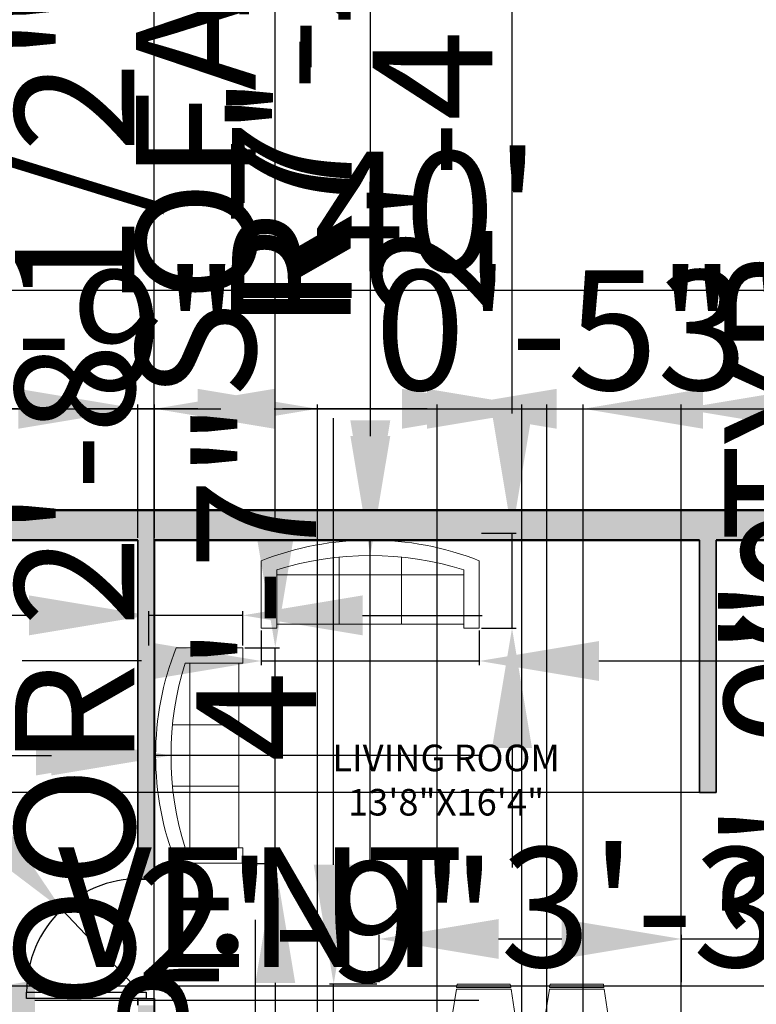
# Model space of a CAD drawing. Units: inches. Extents: x -299 to 1164, y -2 to 940.
# Tile 8 of 11: x 376 to 598, y 490 to 786. Entities that reach past the tile are written whole.
import ezdxf

# ---------------------------------------------------------------- set-up
doc = ezdxf.new("R2010")
doc.units = ezdxf.units.IN
for name, color, linetype, lineweight in [('A-AREA-IDEN', 3, 'Continuous', 25), ('A-FURN', 8, 'Continuous', 18), ('dimensions', 191, 'Continuous', 18), ('doors', 20, 'Continuous', 25), ('inner walls', 7, 'Continuous', 35), ('outer walls', 7, 'Continuous', 50)]:
    doc.layers.add(name, color=color, linetype=linetype, lineweight=lineweight)
doc.layers.add('A-WALL-PATT', color=240, linetype='Continuous', lineweight=13, true_color=0xed1f24)
doc.styles.get("Standard").update_dxf_attribs({"font": 'arial.ttf'})
doc.dimstyles.new('ISO-25', dxfattribs={"dimtxt": 36, "dimasz": 36, "dimexe": 1.25, "dimexo": 0.625, "dimtad": 1, "dimlunit": 3, "dimtxsty": 'Standard', "dimcen": 2.5, "dimazin": 0, "dimtfac": 1, "dimtmove": 0, "dimatfit": 3, "dimfxl": 1, "dimarcsym": 0})

# ---------------------------------------------------------------- blocks, each defined once
blk = doc.blocks.new('Dining Set - 36 x 72 in.')
for p, q in [((-22, 27.5), (-22.1562, 26.50042)), ((-22, 27.5), (-6, 27.5)), ((-5.8437, 26.49966), (-6, 27.5)), ((6, 27.5), (5.8438, 26.50042)), ((6, 27.5), (22, 27.5)), ((22.1563, 26.49966), (22, 27.5)), ((-22.2343, 26.00059), (-23.4847, 17.99762)), ((-22.2304, 26), (-5.7608, 26)), ((-5.8416, 26.5), (-22.1534, 26.5)), ((-4.5152, 17.99762), (-5.7655, 25.99926)), ((5.7657, 26.00059), (4.5153, 17.99762)), ((5.7696, 26), (22.2392, 26)), ((22.1584, 26.5), (5.8466, 26.5)), ((23.4848, 17.99762), (22.2345, 25.99926)), ((36, 18), (-36, 18)), ((-36, 18), (-36, -18)), ((36, -18), (36, 18)), ((-44.0006, 8.23428), (-35.9976, 9.48474)), ((44.0006, 8.23428), (35.9976, 9.48474)), ((-45.5, 8), (-44.5004, 8.15617)), ((-45.5, 8), (-45.5, -8)), ((-44.5, -8.15843), (-44.5, 8.15338)), ((-44, 8.23041), (-44, -8.23915)), ((44, 8.23041), (44, -8.23915)), ((44.5, -8.15843), (44.5, 8.15338)), ((45.5, 8), (44.5005, 8.15617)), ((45.5, 8), (45.5, -8)), ((-44.4997, -8.15631), (-45.5, -8)), ((-35.9976, -9.48476), (-43.9993, -8.2345)), ((35.9976, -9.48476), (43.9993, -8.2345)), ((44.4997, -8.15631), (45.5, -8)), ((-36, -18), (36, -18)), ((-22.2343, -26.0006), (-23.4847, -17.99762)), ((-4.5152, -17.99762), (-5.7655, -25.99928)), ((5.7657, -26.0006), (4.5153, -17.99762)), ((23.4848, -17.99762), (22.2345, -25.99928)), ((-22.2304, -26), (-5.7608, -26)), ((-22, -27.5), (-22.1562, -26.50044)), ((-5.8416, -26.5), (-22.1534, -26.5)), ((-5.8437, -26.49967), (-6, -27.5)), ((5.7696, -26), (22.2392, -26)), ((6, -27.5), (5.8438, -26.50044)), ((22.1584, -26.5), (5.8466, -26.5)), ((22.1563, -26.49967), (22, -27.5)), ((-22, -27.5), (-6, -27.5)), ((6, -27.5), (22, -27.5))]:
    blk.add_line(p, q)
for points in [[(-36, 15), (-31.1772, 14.97754), (-26.8079, 14.91406), (-22.8538, 14.81543), (-19.276, 14.6875), (-16.0362, 14.53613), (-13.0957, 14.36718), (-10.4159, 14.18652), (-7.9583, 14), (-5.6904, 13.81315), (-3.6035, 13.63021), (-1.6954, 13.45508), (0.0365, 13.29166), (1.5945, 13.14388), (2.9811, 13.01562), (4.1988, 12.9108), (5.25, 12.83333), (6.1393, 12.78613), (6.8802, 12.76823), (7.4883, 12.77767), (7.9792, 12.8125), (8.3685, 12.87077), (8.6719, 12.95052), (8.9049, 13.0498), (9.0833, 13.16666), (9.2205, 13.29899), (9.3216, 13.44401), (9.3895, 13.59879), (9.4271, 13.76041), (9.4373, 13.92594), (9.4232, 14.09245), (9.3875, 14.257), (9.3333, 14.41666), (9.2638, 14.56917), (9.1836, 14.71484), (9.0975, 14.85465), (9.0104, 14.98958), (8.9272, 15.1206), (8.8529, 15.2487), (8.7922, 15.37483), (8.75, 15.5), (8.7305, 15.62467), (8.7344, 15.74739), (8.7617, 15.86621), (8.8125, 15.97916), (8.8867, 16.08431), (8.9844, 16.17968), (9.1055, 16.26334), (9.25, 16.33333), (9.4189, 16.38802), (9.6172, 16.42708), (9.8506, 16.45052), (10.125, 16.45833), (10.4463, 16.45052), (10.8203, 16.42708), (11.2529, 16.38802), (11.75, 16.33333), (12.3184, 16.26318), (12.9694, 16.17838), (13.7151, 16.07991), (14.5677, 15.96875), (15.5395, 15.84586), (16.6426, 15.71224), (17.8893, 15.56884), (19.2917, 15.41666), (20.859, 15.25667), (22.5879, 15.08984), (24.4721, 14.91715), (26.5052, 14.73958), (28.6809, 14.5581), (30.9929, 14.3737), (33.4347, 14.18733), (36, 14)], [(-36, 10), (-28.9766, 10.14274), (-23.1725, 10.20442), (-18.4241, 10.19775), (-14.5677, 10.13541), (-11.4399, 10.03011), (-8.877, 9.89453), (-6.7154, 9.74137), (-4.7917, 9.58333), (-2.9698, 9.43082), (-1.2246, 9.28515), (0.4415, 9.14534), (2.026, 9.01041), (3.5266, 8.87939), (4.9408, 8.7513), (6.266, 8.62516), (7.5, 8.5), (8.6411, 8.37549), (9.6914, 8.2539), (10.6538, 8.13818), (11.5312, 8.03125), (12.3267, 7.93603), (13.043, 7.85547), (13.6831, 7.79248), (14.25, 7.75), (14.7471, 7.7303), (15.1797, 7.73307), (15.5537, 7.75732), (15.875, 7.80208), (16.1494, 7.86637), (16.3828, 7.94922), (16.5811, 8.04964), (16.75, 8.16666), (16.8944, 8.29915), (17.0143, 8.44531), (17.1089, 8.60319), (17.1771, 8.77083), (17.218, 8.94629), (17.2305, 9.1276), (17.2137, 9.31282), (17.1667, 9.5), (17.0895, 9.6875), (16.987, 9.875), (16.8649, 10.0625), (16.7292, 10.25), (16.5856, 10.4375), (16.4401, 10.625), (16.2985, 10.8125), (16.1667, 11), (16.05, 11.18733), (15.9518, 11.3737), (15.8752, 11.5581), (15.8229, 11.73958), (15.798, 11.91715), (15.8034, 12.08984), (15.842, 12.25667), (15.9167, 12.41666), (16.0295, 12.56836), (16.1784, 12.70833), (16.3605, 12.83268), (16.5729, 12.9375), (16.8127, 13.01888), (17.0768, 13.07291), (17.3625, 13.0957), (17.6667, 13.08333), (17.9894, 13.03312), (18.3418, 12.94726), (18.7382, 12.82918), (19.1927, 12.68229), (19.7195, 12.51001), (20.3327, 12.31575), (21.0465, 12.10294), (21.875, 11.875), (22.8357, 11.63354), (23.959, 11.37304), (25.2786, 11.08618), (26.8282, 10.76562), (28.6414, 10.40405), (30.752, 9.99414), (33.1936, 9.52856), (36, 9)], [(-36, 5.5), (-30.7157, 5.3348), (-26.069, 5.20963), (-21.9946, 5.11767), (-18.4271, 5.05208), (-15.3009, 5.00602), (-12.5508, 4.97265), (-10.1112, 4.94515), (-7.9167, 4.91666), (-5.909, 4.88167), (-4.0586, 4.83984), (-2.3429, 4.79215), (-0.7396, 4.73958), (0.7739, 4.6831), (2.22, 4.6237), (3.6213, 4.56233), (5, 4.5), (6.373, 4.43782), (7.7344, 4.3776), (9.0723, 4.32129), (10.375, 4.27083), (11.6309, 4.22819), (12.8281, 4.19531), (13.9551, 4.17415), (15, 4.16666), (15.954, 4.17448), (16.819, 4.19791), (17.6001, 4.23698), (18.3021, 4.29166), (18.9299, 4.36198), (19.4883, 4.44791), (19.9823, 4.54948), (20.4167, 4.66666), (20.7969, 4.79899), (21.1302, 4.94401), (21.4245, 5.09879), (21.6875, 5.26041), (21.9271, 5.42594), (22.1511, 5.59245), (22.3672, 5.757), (22.5834, 5.91666), (22.8065, 6.06868), (23.0404, 6.21093), (23.2879, 6.34147), (23.5521, 6.45833), (23.8358, 6.55957), (24.142, 6.64323), (24.4735, 6.70735), (24.8334, 6.75), (25.2235, 6.76969), (25.642, 6.76692), (26.0858, 6.74267), (26.5521, 6.69791), (27.0379, 6.63362), (27.5404, 6.55078), (28.0565, 6.45036), (28.5834, 6.33333), (29.1242, 6.19987), (29.7071, 6.04687), (30.3661, 5.87044), (31.1354, 5.66666), (32.0493, 5.43164), (33.142, 5.16146), (34.4475, 4.85221), (36, 4.5)], [(-36, -1), (-30.7915, -0.6591), (-26.0195, -0.38216), (-21.6519, -0.16284), (-17.6563, 0.00521), (-14.0005, 0.12833), (-10.6523, 0.21289), (-7.5796, 0.26522), (-4.75, 0.29166), (-2.134, 0.29793), (0.2878, 0.28711), (2.5317, 0.26163), (4.6146, 0.22396), (6.5529, 0.17651), (8.3633, 0.12174), (10.0623, 0.06209), (11.6667, 0), (13.1899, -0.06201), (14.6341, -0.1211), (15.9982, -0.17432), (17.2813, -0.21875), (18.4823, -0.25147), (19.6003, -0.26953), (20.6343, -0.27002), (21.5834, -0.25), (22.4481, -0.20768), (23.2357, -0.14584), (23.9549, -0.06836), (24.6146, 0.02083), (25.2235, 0.11784), (25.7904, 0.21875), (26.3241, 0.31966), (26.8334, 0.41666), (27.3265, 0.50618), (27.8099, 0.58593), (28.2894, 0.65397), (28.7709, 0.70833), (29.2601, 0.74707), (29.763, 0.76823), (30.2855, 0.76985), (30.8334, 0.75), (31.4088, 0.70784), (31.9994, 0.64713), (32.589, 0.57275), (33.1615, 0.48958), (33.7008, 0.4025), (34.1908, 0.3164), (34.6153, 0.23616), (34.9584, 0.16666), (35.2099, 0.11165), (35.3848, 0.07031), (35.504, 0.04069), (35.5886, 0.02083), (35.6594, 0.00879), (35.7377, 0.0026), (35.8442, 0.00032), (36, 0)], [(-36, -6.5), (-27.1843, -6.31267), (-20.084, -6.1263), (-14.469, -5.9419), (-10.1094, -5.76042), (-6.7752, -5.58285), (-4.2363, -5.41016), (-2.2629, -5.24333), (-0.625, -5.08334), (0.8708, -4.93099), (2.2715, -4.78646), (3.5872, -4.64974), (4.8281, -4.52084), (6.0046, -4.39974), (7.127, -4.28646), (8.2053, -4.18099), (9.25, -4.08334), (10.2705, -3.99382), (11.2734, -3.91407), (12.2647, -3.84603), (13.25, -3.79167), (14.2354, -3.75293), (15.2266, -3.73177), (16.2295, -3.73015), (17.25, -3.75), (18.2912, -3.79248), (19.3451, -3.85547), (20.4009, -3.93604), (21.4479, -4.03125), (22.4754, -4.13819), (23.4727, -4.25391), (24.4289, -4.37549), (25.3334, -4.5), (26.1785, -4.62492), (26.9694, -4.74935), (27.7145, -4.87281), (28.4219, -4.99479), (29.1, -5.11483), (29.7572, -5.23242), (30.4016, -5.34709), (31.0417, -5.45834), (31.6837, -5.56437), (32.3262, -5.65821), (32.9658, -5.73153), (33.599, -5.77604), (34.2224, -5.78345), (34.8327, -5.74545), (35.4264, -5.65373), (36, -5.5)], [(-36, -10), (-26.4022, -9.81299), (-18.4675, -9.62891), (-11.9839, -9.45069), (-6.7396, -9.28125), (-2.5226, -9.12354), (0.8789, -8.98047), (3.6769, -8.85498), (6.0833, -8.75), (8.2767, -8.66765), (10.3021, -8.60677), (12.1712, -8.56543), (13.8958, -8.54167), (15.4876, -8.53353), (16.9583, -8.53907), (18.3197, -8.55632), (19.5834, -8.58334), (20.7616, -8.61841), (21.8685, -8.66081), (22.9188, -8.71004), (23.9271, -8.76563), (24.9081, -8.82707), (25.8763, -8.89388), (26.8465, -8.96558), (27.8334, -9.04167), (28.8474, -9.12118), (29.8828, -9.20117), (30.93, -9.27824), (31.9792, -9.34896), (33.0205, -9.40991), (34.0443, -9.45768), (35.0407, -9.48885), (36, -9.5)], [(-36, -14.5), (-30.0881, -14.33513), (-25.0332, -14.21224), (-20.7312, -14.12647), (-17.0781, -14.07292), (-13.97, -14.04671), (-11.3027, -14.04297), (-8.9724, -14.05681), (-6.875, -14.08334), (-4.9224, -14.11833), (-3.0905, -14.16016), (-1.3709, -14.20785), (0.2448, -14.26042), (1.7647, -14.3169), (3.1973, -14.3763), (4.5507, -14.43767), (5.8333, -14.5), (7.0554, -14.5621), (8.235, -14.62175), (9.3922, -14.67652), (10.5469, -14.72396), (11.7192, -14.76164), (12.929, -14.78711), (14.1965, -14.79794), (15.5417, -14.79167), (16.9933, -14.76424), (18.6152, -14.70508), (20.4804, -14.60197), (22.6615, -14.44271), (25.2312, -14.21509), (28.2624, -13.9069), (31.8277, -13.50594), (36, -13)]]:
    blk.add_lwpolyline(points)
blk = doc.blocks.new('Sofa - Roundback 7 ft.')
for p, q in [((-12.00002, -32.4421), (-12.00003, -6.5971)), ((11.99997, -32.4421), (11.99998, -6.5971)), ((-36.000027, -34), (-36.000027, -11.4696)), ((-35.999844, -13.3819), (35.9998, -13.3819)), ((35.99998, -34), (35.99998, -11.4696)), ((-36.000027, -32.4421), (35.99998, -32.4421))]:
    blk.add_line(p, q)
for points in [[(-36.000027, -34), (-42.000027, -34), (-42.000027, -8)], [(41.99998, -8), (41.99998, -34), (35.99998, -34)]]:
    blk.add_lwpolyline(points)
for centre, radius, start, end in [((0, -114.25), 114.25, 68.43141, 111.5686), ((-0.00001, -127.1968), 121.1968, 72.72033, 107.2797)]:
    blk.add_arc(centre, radius, start, end)
blk = doc.blocks.new('*D13')
at = {"layer": 'Defpoints', "color": 0, "transparency": 16777216}
for p in [(739.07, 704.71), (259.07, 638.49), (739.07, 638.49)]:
    blk.add_point(p, dxfattribs=at)
at = {"layer": 'dimensions', "color": 0, "lineweight": -2, "transparency": 16777216}
for p, q in [((259.07, 639.11), (259.07, 705.96)), ((739.07, 639.11), (739.07, 705.96)), ((295.07, 704.71), (703.07, 704.71))]:
    blk.add_line(p, q, dxfattribs=at)
at = {"layer": 'dimensions', "color": 0, "transparency": 16777216}
for points in [[(295.07, 710.71), (295.07, 698.71), (259.07, 704.71)], [(703.07, 710.71), (703.07, 698.71), (739.07, 704.71)]]:
    blk.add_solid(points, dxfattribs=at)
at = {"layer": 'dimensions', "color": 0, "transparency": 16777216, "insert": (499.07, 723.71), "char_height": 36, "attachment_point": 5}
blk.add_mtext("40'", dxfattribs=at)
blk = doc.blocks.new('DOOR-36IN')
blk.add_lwpolyline([(0, 36), (2, 36), (2, 0), (0, 0)], close=True)
blk.add_arc((2.32, 2.25), 33.75, 356.1776, 90.5492)
blk = doc.blocks.new('*D19')
at = {"layer": 'Defpoints', "color": 0, "transparency": 16777216}
for p in [(449.18, 602.94), (514.78, 602.94), (514.78, 593.1)]:
    blk.add_point(p, dxfattribs=at)
at = {"layer": 'dimensions', "color": 0, "lineweight": -2, "transparency": 16777216}
for p, q in [((449.18, 602.31), (449.18, 591.85)), ((514.78, 602.31), (514.78, 591.85)), ((413.18, 593.1), (377.18, 593.1)), ((449.18, 593.1), (514.78, 593.1)), ((550.78, 593.1), (918.34, 593.1))]:
    blk.add_line(p, q, dxfattribs=at)
at = {"layer": 'dimensions', "color": 0, "transparency": 16777216}
for points in [[(413.18, 599.1), (413.18, 587.1), (449.18, 593.1)], [(550.78, 599.1), (550.78, 587.1), (514.78, 593.1)]]:
    blk.add_solid(points, dxfattribs=at)
at = {"layer": 'dimensions', "color": 0, "transparency": 16777216, "insert": (752.56, 612.35), "char_height": 36, "attachment_point": 5}
blk.add_mtext('SOFA 5\'-5 1/2"', dxfattribs=at)
blk = doc.blocks.new('*D20')
at = {"layer": 'Defpoints', "color": 0, "transparency": 16777216}
for p in [(514.78, 631.57), (524.62, 631.57), (514.78, 602.94)]:
    blk.add_point(p, dxfattribs=at)
at = {"layer": 'dimensions', "color": 0, "lineweight": -2, "transparency": 16777216}
for p, q in [((524.62, 667.57), (524.62, 885.02)), ((515.4, 631.57), (525.87, 631.57)), ((524.62, 602.94), (524.62, 631.57)), ((515.4, 602.94), (525.87, 602.94)), ((524.62, 566.94), (524.62, 530.94))]:
    blk.add_line(p, q, dxfattribs=at)
at = {"layer": 'dimensions', "color": 0, "transparency": 16777216}
for points in [[(518.62, 667.57), (530.62, 667.57), (524.62, 631.57)], [(518.62, 566.94), (530.62, 566.94), (524.62, 602.94)]]:
    blk.add_solid(points, dxfattribs=at)
at = {"layer": 'dimensions', "color": 0, "transparency": 16777216, "insert": (505.38, 794.29), "char_height": 36, "attachment_point": 5, "rotation": 90}
blk.add_mtext('2\'-4 1/2"', dxfattribs=at)
blk = doc.blocks.new('*D25')
at = {"layer": 'Defpoints', "color": 0, "transparency": 16777216}
for p in [(443.65, 597.1), (453.38, 597.1), (443.65, 532.21)]:
    blk.add_point(p, dxfattribs=at)
at = {"layer": 'dimensions', "color": 0, "lineweight": -2, "transparency": 16777216}
for p, q in [((453.38, 633.1), (453.38, 916.77)), ((444.27, 597.1), (454.63, 597.1)), ((453.38, 532.21), (453.38, 597.1)), ((444.27, 532.21), (454.63, 532.21)), ((453.38, 496.21), (453.38, 460.21))]:
    blk.add_line(p, q, dxfattribs=at)
at = {"layer": 'dimensions', "color": 0, "transparency": 16777216}
for points in [[(447.38, 633.1), (459.38, 633.1), (453.38, 597.1)], [(447.38, 496.21), (459.38, 496.21), (453.38, 532.21)]]:
    blk.add_solid(points, dxfattribs=at)
at = {"layer": 'dimensions', "color": 0, "transparency": 16777216, "insert": (434.13, 792.94), "char_height": 36, "attachment_point": 5, "rotation": 90}
blk.add_mtext('SOFA 5\'-5"', dxfattribs=at)
blk = doc.blocks.new('*D26')
at = {"layer": 'Defpoints', "color": 0, "transparency": 16777216}
for p in [(415.32, 606.83), (415.32, 597.1), (443.65, 597.1)]:
    blk.add_point(p, dxfattribs=at)
at = {"layer": 'dimensions', "color": 0, "lineweight": -2, "transparency": 16777216}
for p, q in [((415.32, 597.72), (415.32, 608.08)), ((443.65, 597.72), (443.65, 608.08)), ((379.32, 606.83), (161.88, 606.83)), ((443.65, 606.83), (415.32, 606.83)), ((479.65, 606.83), (515.65, 606.83))]:
    blk.add_line(p, q, dxfattribs=at)
at = {"layer": 'dimensions', "color": 0, "transparency": 16777216}
for points in [[(379.32, 612.83), (379.32, 600.83), (415.32, 606.83)], [(479.65, 612.83), (479.65, 600.83), (443.65, 606.83)]]:
    blk.add_solid(points, dxfattribs=at)
at = {"layer": 'dimensions', "color": 0, "transparency": 16777216, "insert": (252.6, 626.07), "char_height": 36, "attachment_point": 5}
blk.add_mtext('2\'-4 1/2"', dxfattribs=at)
blk = doc.blocks.new('*D27')
at = {"layer": 'Defpoints', "color": 0, "transparency": 16777216}
for p in [(412.07, 375.49), (416.95, 375.49), (412.07, 342.99)]:
    blk.add_point(p, dxfattribs=at)
at = {"layer": 'dimensions', "color": 0, "lineweight": -2, "transparency": 16777216}
for p, q in [((416.95, 411.49), (416.95, 915.12)), ((412.7, 375.49), (418.2, 375.49)), ((416.95, 342.99), (416.95, 375.49)), ((412.7, 342.99), (418.2, 342.99)), ((416.95, 306.99), (416.95, 270.99))]:
    blk.add_line(p, q, dxfattribs=at)
at = {"layer": 'dimensions', "color": 0, "transparency": 16777216}
for points in [[(410.95, 411.49), (422.95, 411.49), (416.95, 375.49)], [(410.95, 306.99), (422.95, 306.99), (416.95, 342.99)]]:
    blk.add_solid(points, dxfattribs=at)
at = {"layer": 'dimensions', "color": 0, "transparency": 16777216, "insert": (397.69, 681.3), "char_height": 36, "attachment_point": 5, "rotation": 90}
blk.add_mtext('DOOR 2\'-8 1/2" TYP.', dxfattribs=at)
blk = doc.blocks.new('*D32')
at = {"layer": 'Defpoints', "color": 0, "transparency": 16777216}
for p in [(348.07, 310.2), (360.07, 310.2), (348.07, 250.2)]:
    blk.add_point(p, dxfattribs=at)
at = {"layer": 'dimensions', "color": 0, "lineweight": -2, "transparency": 16777216}
for p, q in [((360.07, 346.2), (360.07, 602.89)), ((348.7, 310.2), (361.32, 310.2)), ((360.07, 250.2), (360.07, 310.2)), ((348.7, 250.2), (361.32, 250.2)), ((360.07, 214.2), (360.07, 178.2))]:
    blk.add_line(p, q, dxfattribs=at)
at = {"layer": 'dimensions', "color": 0, "transparency": 16777216}
for points in [[(354.07, 346.2), (366.07, 346.2), (360.07, 310.2)], [(354.07, 214.2), (366.07, 214.2), (360.07, 250.2)]]:
    blk.add_solid(points, dxfattribs=at)
at = {"layer": 'dimensions', "color": 0, "transparency": 16777216, "insert": (341.07, 492.55), "char_height": 36, "attachment_point": 5, "rotation": 90}
blk.add_mtext('5\'-0" TYP.', dxfattribs=at)
blk = doc.blocks.new('*D34')
at = {"layer": 'Defpoints', "color": 0, "transparency": 16777216}
for p in [(443.84, 222.49), (447.44, 222.49), (443.84, 213.49)]:
    blk.add_point(p, dxfattribs=at)
at = {"layer": 'dimensions', "color": 0, "lineweight": -2, "transparency": 16777216}
for p, q in [((447.44, 258.49), (447.44, 515.18)), ((444.47, 222.49), (448.69, 222.49)), ((447.44, 213.49), (447.44, 222.49)), ((444.47, 213.49), (448.69, 213.49)), ((447.44, 177.49), (447.44, 141.49))]:
    blk.add_line(p, q, dxfattribs=at)
at = {"layer": 'dimensions', "color": 0, "transparency": 16777216}
for points in [[(441.44, 258.49), (453.44, 258.49), (447.44, 222.49)], [(441.44, 177.49), (453.44, 177.49), (447.44, 213.49)]]:
    blk.add_solid(points, dxfattribs=at)
at = {"layer": 'dimensions', "color": 0, "transparency": 16777216, "insert": (428.44, 404.83), "char_height": 36, "attachment_point": 5, "rotation": 90}
blk.add_mtext('0\'-9" TYP.', dxfattribs=at)
blk = doc.blocks.new('*D35')
at = {"layer": 'Defpoints', "color": 0, "transparency": 16777216}
for p in [(307.07, 495.34), (268.07, 489.49), (307.07, 489.49)]:
    blk.add_point(p, dxfattribs=at)
at = {"layer": 'dimensions', "color": 0, "lineweight": -2, "transparency": 16777216}
for p, q in [((232.07, 495.34), (196.07, 495.34)), ((268.07, 490.11), (268.07, 496.59)), ((268.07, 495.34), (307.07, 495.34)), ((307.07, 490.11), (307.07, 496.59)), ((343.07, 495.34), (749.73, 495.34))]:
    blk.add_line(p, q, dxfattribs=at)
at = {"layer": 'dimensions', "color": 0, "transparency": 16777216}
for points in [[(232.07, 501.34), (232.07, 489.34), (268.07, 495.34)], [(343.07, 501.34), (343.07, 489.34), (307.07, 495.34)]]:
    blk.add_solid(points, dxfattribs=at)
at = {"layer": 'dimensions', "color": 0, "transparency": 16777216, "insert": (564.4, 514.36), "char_height": 36, "attachment_point": 5}
blk.add_mtext('VENT 3\'-3" TYP.', dxfattribs=at)
blk = doc.blocks.new('*D37')
at = {"layer": 'Defpoints', "color": 0, "transparency": 16777216}
for p in [(588.07, 400.99), (624.7, 400.99), (624.7, 395.5)]:
    blk.add_point(p, dxfattribs=at)
at = {"layer": 'dimensions', "color": 0, "lineweight": -2, "transparency": 16777216}
for p, q in [((588.07, 400.36), (588.07, 394.25)), ((624.7, 400.36), (624.7, 394.25)), ((552.07, 395.5), (516.07, 395.5)), ((588.07, 395.5), (624.7, 395.5)), ((660.7, 395.5), (1164.33, 395.5))]:
    blk.add_line(p, q, dxfattribs=at)
at = {"layer": 'dimensions', "color": 0, "transparency": 16777216}
for points in [[(552.07, 401.5), (552.07, 389.5), (588.07, 395.5)], [(660.7, 401.5), (660.7, 389.5), (624.7, 395.5)]]:
    blk.add_solid(points, dxfattribs=at)
at = {"layer": 'dimensions', "color": 0, "transparency": 16777216, "insert": (930.51, 414.76), "char_height": 36, "attachment_point": 5}
blk.add_mtext('DOOR 3\'-0 1/2" TYP.', dxfattribs=at)
blk = doc.blocks.new('*D38')
at = {"layer": 'Defpoints', "color": 0, "transparency": 16777216}
for p in [(624.7, 437.08), (630.19, 437.08), (624.7, 400.99)]:
    blk.add_point(p, dxfattribs=at)
at = {"layer": 'dimensions', "color": 0, "lineweight": -2, "transparency": 16777216}
for p, q in [((630.19, 473.08), (630.19, 729.74)), ((625.32, 437.08), (631.44, 437.08)), ((630.19, 400.99), (630.19, 437.08)), ((625.32, 400.99), (631.44, 400.99)), ((630.19, 364.99), (630.19, 328.99))]:
    blk.add_line(p, q, dxfattribs=at)
at = {"layer": 'dimensions', "color": 0, "transparency": 16777216}
for points in [[(624.19, 473.08), (636.19, 473.08), (630.19, 437.08)], [(624.19, 364.99), (636.19, 364.99), (630.19, 400.99)]]:
    blk.add_solid(points, dxfattribs=at)
at = {"layer": 'dimensions', "color": 0, "transparency": 16777216, "insert": (611.17, 619.41), "char_height": 36, "attachment_point": 5, "rotation": 90}
blk.add_mtext('3\'-0" TYP.', dxfattribs=at)
blk = doc.blocks.new('*D39')
at = {"layer": 'Defpoints', "color": 0, "transparency": 16777216}
for p in [(575.6, 509.45), (484.6, 495.8), (575.6, 495.8)]:
    blk.add_point(p, dxfattribs=at)
at = {"layer": 'dimensions', "color": 0, "lineweight": -2, "transparency": 16777216}
for p, q in [((484.6, 496.43), (484.6, 510.7)), ((575.6, 496.43), (575.6, 510.7)), ((520.6, 509.45), (539.6, 509.45)), ((575.6, 509.45), (1008.53, 509.45))]:
    blk.add_line(p, q, dxfattribs=at)
at = {"layer": 'dimensions', "color": 0, "transparency": 16777216}
for points in [[(520.6, 515.45), (520.6, 503.45), (484.6, 509.45)], [(539.6, 515.45), (539.6, 503.45), (575.6, 509.45)]]:
    blk.add_solid(points, dxfattribs=at)
at = {"layer": 'dimensions', "color": 0, "transparency": 16777216, "insert": (810.07, 528.69), "char_height": 36, "attachment_point": 5}
blk.add_mtext('DINING SET 7\'-7"', dxfattribs=at)
blk = doc.blocks.new('*D40')
at = {"layer": 'Defpoints', "color": 0, "transparency": 16777216}
for p in [(470.95, 495.8), (484.6, 495.8), (484.6, 440.8)]:
    blk.add_point(p, dxfattribs=at)
at = {"layer": 'dimensions', "color": 0, "lineweight": -2, "transparency": 16777216}
for p, q in [((470.95, 531.8), (470.95, 666.2)), ((483.98, 495.8), (469.7, 495.8)), ((470.95, 440.8), (470.95, 495.8)), ((483.98, 440.8), (469.7, 440.8)), ((470.95, 404.8), (470.95, 368.8))]:
    blk.add_line(p, q, dxfattribs=at)
at = {"layer": 'dimensions', "color": 0, "transparency": 16777216}
for points in [[(464.95, 531.8), (476.95, 531.8), (470.95, 495.8)], [(464.95, 404.8), (476.95, 404.8), (470.95, 440.8)]]:
    blk.add_solid(points, dxfattribs=at)
at = {"layer": 'dimensions', "color": 0, "transparency": 16777216, "insert": (452.33, 617), "char_height": 36, "attachment_point": 5, "rotation": 90}
blk.add_mtext('4\'-7"', dxfattribs=at)
blk = doc.blocks.new('*D43')
at = {"layer": 'Defpoints', "color": 0, "transparency": 16777216}
for p in [(268.07, 668.99), (259.07, 638.49), (268.07, 629.49)]:
    blk.add_point(p, dxfattribs=at)
at = {"layer": 'dimensions', "color": 0, "lineweight": -2, "transparency": 16777216}
for p, q in [((259.07, 639.11), (259.07, 670.24)), ((268.07, 630.11), (268.07, 670.24)), ((223.07, 668.99), (187.07, 668.99)), ((259.07, 668.99), (268.07, 668.99)), ((304.07, 668.99), (437.02, 668.99))]:
    blk.add_line(p, q, dxfattribs=at)
at = {"layer": 'dimensions', "color": 0, "transparency": 16777216}
for points in [[(223.07, 674.99), (223.07, 662.99), (259.07, 668.99)], [(304.07, 674.99), (304.07, 662.99), (268.07, 668.99)]]:
    blk.add_solid(points, dxfattribs=at)
at = {"layer": 'dimensions', "color": 0, "transparency": 16777216, "insert": (388.54, 687.99), "char_height": 36, "attachment_point": 5}
blk.add_mtext('0\'-9"', dxfattribs=at)
blk = doc.blocks.new('*D44')
at = {"layer": 'Defpoints', "color": 0, "transparency": 16777216}
for p in [(417.07, 668.99), (412.07, 629.49), (417.07, 629.49)]:
    blk.add_point(p, dxfattribs=at)
at = {"layer": 'dimensions', "color": 0, "lineweight": -2, "transparency": 16777216}
for p, q in [((412.07, 630.11), (412.07, 670.24)), ((417.07, 630.11), (417.07, 670.24)), ((376.07, 668.99), (340.07, 668.99)), ((412.07, 668.99), (417.07, 668.99)), ((453.07, 668.99), (586.02, 668.99))]:
    blk.add_line(p, q, dxfattribs=at)
at = {"layer": 'dimensions', "color": 0, "transparency": 16777216}
for points in [[(376.07, 674.99), (376.07, 662.99), (412.07, 668.99)], [(453.07, 674.99), (453.07, 662.99), (417.07, 668.99)]]:
    blk.add_solid(points, dxfattribs=at)
at = {"layer": 'dimensions', "color": 0, "transparency": 16777216, "insert": (537.54, 687.99), "char_height": 36, "attachment_point": 5}
blk.add_mtext('0\'-5"', dxfattribs=at)
blk = doc.blocks.new('*D47')
at = {"layer": 'Defpoints', "color": 0, "transparency": 16777216}
for p in [(502.07, 668.99), (466.07, 222.49), (502.07, 222.49)]:
    blk.add_point(p, dxfattribs=at)
at = {"layer": 'dimensions', "color": 0, "lineweight": -2, "transparency": 16777216}
for p, q in [((466.07, 223.11), (466.07, 670.24)), ((502.07, 223.11), (502.07, 670.24)), ((430.07, 668.99), (394.07, 668.99)), ((466.07, 668.99), (502.07, 668.99)), ((538.07, 668.99), (670.99, 668.99))]:
    blk.add_line(p, q, dxfattribs=at)
at = {"layer": 'dimensions', "color": 0, "transparency": 16777216}
for points in [[(430.07, 674.99), (430.07, 662.99), (466.07, 668.99)], [(538.07, 674.99), (538.07, 662.99), (502.07, 668.99)]]:
    blk.add_solid(points, dxfattribs=at)
at = {"layer": 'dimensions', "color": 0, "transparency": 16777216, "insert": (622.53, 688.01), "char_height": 36, "attachment_point": 5}
blk.add_mtext('3\'-0"', dxfattribs=at)
blk = doc.blocks.new('*D48')
at = {"layer": 'Defpoints', "color": 0, "transparency": 16777216}
for p in [(546.07, 668.99), (535.07, 222.49), (546.07, 222.49)]:
    blk.add_point(p, dxfattribs=at)
at = {"layer": 'dimensions', "color": 0, "lineweight": -2, "transparency": 16777216}
for p, q in [((535.07, 223.11), (535.07, 670.24)), ((546.07, 223.11), (546.07, 670.24)), ((499.07, 668.99), (463.07, 668.99)), ((535.07, 668.99), (546.07, 668.99)), ((582.07, 668.99), (742.99, 668.99))]:
    blk.add_line(p, q, dxfattribs=at)
at = {"layer": 'dimensions', "color": 0, "transparency": 16777216}
for points in [[(499.07, 674.99), (499.07, 662.99), (535.07, 668.99)], [(582.07, 674.99), (582.07, 662.99), (546.07, 668.99)]]:
    blk.add_solid(points, dxfattribs=at)
at = {"layer": 'dimensions', "color": 0, "transparency": 16777216, "insert": (680.53, 687.99), "char_height": 36, "attachment_point": 5}
blk.add_mtext('0\'-11"', dxfattribs=at)
blk = doc.blocks.new('*D52')
at = {"layer": 'Defpoints', "color": 0, "transparency": 16777216}
for p in [(575.54, 668.99), (527.54, 311.49), (575.54, 311.49)]:
    blk.add_point(p, dxfattribs=at)
at = {"layer": 'dimensions', "color": 0, "lineweight": -2, "transparency": 16777216}
for p, q in [((527.54, 312.11), (527.54, 670.24)), ((575.54, 312.11), (575.54, 670.24)), ((491.54, 668.99), (455.54, 668.99)), ((527.54, 668.99), (575.54, 668.99)), ((611.54, 668.99), (745.94, 668.99))]:
    blk.add_line(p, q, dxfattribs=at)
at = {"layer": 'dimensions', "color": 0, "transparency": 16777216}
for points in [[(491.54, 674.99), (491.54, 662.99), (527.54, 668.99)], [(611.54, 674.99), (611.54, 662.99), (575.54, 668.99)]]:
    blk.add_solid(points, dxfattribs=at)
at = {"layer": 'dimensions', "color": 0, "transparency": 16777216, "insert": (696.74, 687.99), "char_height": 36, "attachment_point": 5}
blk.add_mtext('4\'-0"', dxfattribs=at)
blk = doc.blocks.new('*D53')
at = {"layer": 'Defpoints', "color": 0, "transparency": 16777216}
for p in [(177.57, 553.49), (586.07, 553.49), (586.07, 481.49)]:
    blk.add_point(p, dxfattribs=at)
at = {"layer": 'dimensions', "color": 0, "lineweight": -2, "transparency": 16777216}
for p, q in [((177.57, 589.49), (177.57, 722.63)), ((585.45, 553.49), (176.32, 553.49)), ((177.57, 481.49), (177.57, 553.49)), ((585.45, 481.49), (176.32, 481.49)), ((177.57, 445.49), (177.57, 409.49))]:
    blk.add_line(p, q, dxfattribs=at)
at = {"layer": 'dimensions', "color": 0, "transparency": 16777216}
for points in [[(171.57, 589.49), (183.57, 589.49), (177.57, 553.49)], [(171.57, 445.49), (183.57, 445.49), (177.57, 481.49)]]:
    blk.add_solid(points, dxfattribs=at)
at = {"layer": 'dimensions', "color": 0, "transparency": 16777216, "insert": (158.57, 674.06), "char_height": 36, "attachment_point": 5, "rotation": 90}
blk.add_mtext('6\'-0"', dxfattribs=at)
blk = doc.blocks.new('*D54')
at = {"layer": 'Defpoints', "color": 0, "transparency": 16777216}
for p in [(345.07, 490.99), (312.07, 460.49), (345.07, 460.49)]:
    blk.add_point(p, dxfattribs=at)
at = {"layer": 'dimensions', "color": 0, "lineweight": -2, "transparency": 16777216}
for p, q in [((312.07, 461.11), (312.07, 492.24)), ((345.07, 461.11), (345.07, 492.24)), ((276.07, 490.99), (240.07, 490.99)), ((312.07, 490.99), (345.07, 490.99)), ((381.07, 490.99), (514.63, 490.99))]:
    blk.add_line(p, q, dxfattribs=at)
at = {"layer": 'dimensions', "color": 0, "transparency": 16777216}
for points in [[(276.07, 496.99), (276.07, 484.99), (312.07, 490.99)], [(381.07, 496.99), (381.07, 484.99), (345.07, 490.99)]]:
    blk.add_solid(points, dxfattribs=at)
at = {"layer": 'dimensions', "color": 0, "transparency": 16777216, "insert": (465.85, 509.99), "char_height": 36, "attachment_point": 5}
blk.add_mtext('2\'-9"', dxfattribs=at)
blk = doc.blocks.new('*D58')
at = {"layer": 'Defpoints', "color": 0, "transparency": 16777216}
for p in [(456.35, 347.49), (770.93, 347.49), (456.35, 311.49)]:
    blk.add_point(p, dxfattribs=at)
at = {"layer": 'dimensions', "color": 0, "lineweight": -2, "transparency": 16777216}
for p, q in [((770.93, 383.49), (770.93, 516.41)), ((456.97, 347.49), (772.18, 347.49)), ((770.93, 311.49), (770.93, 347.49)), ((456.97, 311.49), (772.18, 311.49)), ((770.93, 275.49), (770.93, 239.49))]:
    blk.add_line(p, q, dxfattribs=at)
at = {"layer": 'dimensions', "color": 0, "transparency": 16777216}
for points in [[(764.93, 383.49), (776.93, 383.49), (770.93, 347.49)], [(764.93, 275.49), (776.93, 275.49), (770.93, 311.49)]]:
    blk.add_solid(points, dxfattribs=at)
at = {"layer": 'dimensions', "color": 0, "transparency": 16777216, "insert": (751.91, 467.95), "char_height": 36, "attachment_point": 5, "rotation": 90}
blk.add_mtext('3\'-0"', dxfattribs=at)
blk = doc.blocks.new('*D61')
at = {"layer": 'Defpoints', "color": 0, "transparency": 16777216}
for p in [(389.15, 518.35), (412.32, 493.81)]:
    blk.add_point(p, dxfattribs=at)
at = {"layer": 'dimensions', "color": 0, "lineweight": -2, "transparency": 16777216}
for p, q in [((176.74, 743.24), (364.43, 544.52)), ((412.32, 493.81), (389.15, 518.35))]:
    blk.add_line(p, q, dxfattribs=at)
at = {"layer": 'dimensions', "color": 0, "transparency": 16777216}
blk.add_solid([(368.79, 548.64), (360.07, 540.4), (389.15, 518.35)], dxfattribs=at)
at = {"layer": 'dimensions', "color": 0, "transparency": 16777216, "insert": (272.04, 670.02), "char_height": 36, "attachment_point": 5, "rotation": 313.3644}
blk.add_mtext('2X R2\'-10"', dxfattribs=at)
blk = doc.blocks.new('*D63')
at = {"layer": 'Defpoints', "color": 0, "transparency": 16777216}
for p in [(658.07, 623.87), (658.07, 510.33)]:
    blk.add_point(p, dxfattribs=at)
at = {"layer": 'dimensions', "color": 0, "lineweight": -2, "transparency": 16777216}
for p, q in [((658.07, 911.15), (658.07, 659.87)), ((658.07, 510.33), (658.07, 623.87))]:
    blk.add_line(p, q, dxfattribs=at)
at = {"layer": 'dimensions', "color": 0, "transparency": 16777216}
blk.add_solid([(652.07, 659.87), (664.07, 659.87), (658.07, 623.87)], dxfattribs=at)
at = {"layer": 'dimensions', "color": 0, "transparency": 16777216, "insert": (638.83, 803.51), "char_height": 36, "attachment_point": 5, "rotation": 90}
blk.add_mtext('R9\'-5 1/2"', dxfattribs=at)
blk = doc.blocks.new('*D67')
at = {"layer": 'Defpoints', "color": 0, "transparency": 16777216}
for p in [(481.98, 624.8), (481.98, 530.15)]:
    blk.add_point(p, dxfattribs=at)
at = {"layer": 'dimensions', "color": 0, "lineweight": -2, "transparency": 16777216}
for p, q in [((481.98, 940.06), (481.98, 660.8)), ((481.98, 530.15), (481.98, 624.8))]:
    blk.add_line(p, q, dxfattribs=at)
at = {"layer": 'dimensions', "color": 0, "transparency": 16777216}
blk.add_solid([(475.98, 660.8), (487.98, 660.8), (481.98, 624.8)], dxfattribs=at)
at = {"layer": 'dimensions', "color": 0, "transparency": 16777216, "insert": (462.74, 818.43), "char_height": 36, "attachment_point": 5, "rotation": 90}
blk.add_mtext('R7\'-10 1/2"', dxfattribs=at)
blk = doc.blocks.new('*D68')
at = {"layer": 'Defpoints', "color": 0, "transparency": 16777216}
for p in [(422.02, 564.66), (515.63, 564.66)]:
    blk.add_point(p, dxfattribs=at)
at = {"layer": 'dimensions', "color": 0, "lineweight": -2, "transparency": 16777216}
for p, q in [((134.73, 564.66), (386.02, 564.66)), ((515.63, 564.66), (422.02, 564.66))]:
    blk.add_line(p, q, dxfattribs=at)
at = {"layer": 'dimensions', "color": 0, "transparency": 16777216}
blk.add_solid([(386.02, 570.66), (386.02, 558.66), (422.02, 564.66)], dxfattribs=at)
at = {"layer": 'dimensions', "color": 0, "transparency": 16777216, "insert": (242.37, 583.9), "char_height": 36, "attachment_point": 5, "rotation": 359.9997}
blk.add_mtext('R7\'-9 1/2"', dxfattribs=at)
blk = doc.blocks.new('*D69')
at = {"layer": 'Defpoints', "color": 0, "transparency": 16777216}
for p in [(481.98, 629.49), (481.98, 540.26)]:
    blk.add_point(p, dxfattribs=at)
at = {"layer": 'dimensions', "color": 0, "lineweight": -2, "transparency": 16777216}
for p, q in [((481.98, 832.89), (481.98, 665.49)), ((481.98, 540.26), (481.98, 629.49))]:
    blk.add_line(p, q, dxfattribs=at)
at = {"layer": 'dimensions', "color": 0, "transparency": 16777216}
blk.add_solid([(475.98, 665.49), (487.98, 665.49), (481.98, 629.49)], dxfattribs=at)
at = {"layer": 'dimensions', "color": 0, "transparency": 16777216, "insert": (463.05, 767.19), "char_height": 36, "attachment_point": 5, "rotation": 90}
blk.add_mtext('R7\'-5"', dxfattribs=at)
blk = doc.blocks.new('*D70')
at = {"layer": 'Defpoints', "color": 0, "transparency": 16777216}
for p in [(417.38, 564.66), (505.63, 564.66)]:
    blk.add_point(p, dxfattribs=at)
at = {"layer": 'dimensions', "color": 0, "lineweight": -2, "transparency": 16777216}
for p, q in [((130.1, 564.66), (381.38, 564.66)), ((505.63, 564.66), (417.38, 564.66))]:
    blk.add_line(p, q, dxfattribs=at)
at = {"layer": 'dimensions', "color": 0, "transparency": 16777216}
blk.add_solid([(381.38, 570.66), (381.38, 558.66), (417.38, 564.66)], dxfattribs=at)
at = {"layer": 'dimensions', "color": 0, "transparency": 16777216, "insert": (237.74, 583.9), "char_height": 36, "attachment_point": 5, "rotation": 359.9997}
blk.add_mtext('R7\'-4 1/2"', dxfattribs=at)

msp = doc.modelspace()

# ---------------------------------------------------------------- hatches: boundary and pattern name
at = {"layer": 'A-WALL-PATT'}
h = msp.add_hatch(color=256, dxfattribs=at)
h.dxf.hatch_style = 1
h.paths.add_polyline_path([(312.071, 460.489), (307.071, 460.489), (307.071, 432.489), (307.071, 427.489), (372.071, 427.489), (372.071, 375.489), (372.071, 370.489), (380.071, 370.489, -0.0217424), (380.071, 372.989), (380.071, 375.489), (377.071, 375.489), (377.071, 427.489), (417.071, 427.489), (417.071, 489.489), (412.071, 489.489), (412.071, 484.489), (412.071, 432.489), (312.071, 432.489)], flags=17)
h.paths.add_polyline_path([(340.071, 372.989, -0.0217424), (340.071, 375.489), (268.071, 375.489), (268.071, 427.489), (268.071, 432.489), (268.071, 484.489), (268.071, 489.489), (268.071, 629.489), (412.071, 629.489), (412.071, 527.563, -0.0185322), (414.571, 527.489), (417.071, 527.489), (417.071, 629.489), (581.071, 629.489), (581.071, 553.489), (586.071, 553.489), (586.071, 629.489), (730.071, 629.489), (730.071, 405.489), (713.071, 405.489), (713.071, 396.489), (739.071, 396.489), (739.071, 638.489), (259.071, 638.489), (259.071, 183.489), (304.071, 183.489), (304.071, 192.489), (268.071, 192.489), (268.071, 370.489), (340.071, 370.489)])
h.paths.add_polyline_path([(417.071, 188.489), (417.071, 213.489), (461.071, 213.489), (461.071, 188.489)], flags=16)
h.paths.add_polyline_path([(586.071, 313.578), (577.071, 313.578), (577.071, 311.489), (575.54, 311.489), (575.54, 302.489), (586.071, 302.489)], flags=16)
h.paths.add_polyline_path([(586.071, 405.489), (586.071, 481.489), (581.071, 481.489), (581.071, 432.489), (499.071, 432.489), (499.071, 427.489), (577.071, 427.489), (577.071, 385.578), (586.071, 385.578), (586.071, 396.489)], flags=17)
h.paths.add_polyline_path([(641.071, 405.489), (624.071, 405.489, -0.0333689), (624.071, 400.989), (624.071, 396.489), (641.071, 396.489)], flags=17)
h.paths.add_polyline_path([(491.866, 222.489), (491.866, 213.489), (586.071, 213.489), (586.071, 222.489)])
edge = h.paths.add_edge_path()
edge.add_line((467.866, 213.489), (467.866, 222.489))
edge.add_line((467.866, 222.489), (466.071, 222.489))
edge.add_line((466.071, 222.489), (466.071, 302.489))
edge.add_line((466.071, 302.489), (527.54, 302.489))
edge.add_line((527.54, 302.489), (527.54, 311.489))
edge.add_line((527.54, 311.489), (449.071, 311.489))
edge.add_line((449.071, 311.489), (449.071, 308.989))
edge.add_arc((420.339, 307.739), 28.759, -2.4911, 2.4911, ccw=False)
edge.add_line((449.071, 306.489), (461.071, 306.489))
edge.add_line((461.071, 306.489), (461.071, 222.489))
edge.add_line((461.071, 222.489), (443.844, 222.489))
edge.add_line((443.844, 222.489), (443.844, 213.489))
edge.add_line((443.844, 213.489), (419.844, 213.489))
edge.add_line((419.844, 213.489), (419.844, 222.489))
edge.add_line((419.844, 222.489), (417.071, 222.489))
edge.add_line((417.071, 222.489), (417.071, 306.489))
edge.add_line((417.071, 306.489), (417.071, 311.489))
edge.add_line((417.071, 311.489), (417.071, 375.489))
edge.add_line((417.071, 375.489), (412.071, 375.489))
edge.add_line((412.071, 375.489), (412.071, 370.489))
edge.add_line((412.071, 370.489), (412.071, 192.489))
edge.add_line((412.071, 192.489), (376.071, 192.489))
edge.add_line((376.071, 192.489), (376.071, 183.489))
edge.add_line((376.071, 183.489), (412.071, 183.489))
edge.add_line((412.071, 183.489), (466.071, 183.489))
edge.add_line((466.071, 183.489), (466.071, 213.489))
edge.add_line((466.071, 213.489), (467.866, 213.489))

# ---------------------------------------------------------------- linework, layer by layer
at = {"layer": 'doors'}
for p, q in [((412.071, 527.489), (417.071, 527.489)), ((412.071, 491.489), (417.071, 491.489))]:
    msp.add_line(p, q, dxfattribs=at)
at = {"layer": 'inner walls'}
for p, q in [((412.071, 629.489), (412.071, 527.489)), ((417.071, 629.489), (417.071, 527.489)), ((581.071, 629.489), (581.071, 553.489)), ((586.071, 629.489), (586.071, 553.489)), ((586.071, 553.489), (581.071, 553.489)), ((412.071, 491.489), (412.071, 489.489)), ((417.071, 491.489), (417.071, 427.489))]:
    msp.add_line(p, q, dxfattribs=at)
at = {"layer": 'outer walls'}
for p, q in [((739.071, 638.489), (259.071, 638.489)), ((412.071, 629.489), (268.071, 629.489)), ((581.071, 629.489), (417.071, 629.489)), ((730.071, 629.489), (586.071, 629.489))]:
    msp.add_line(p, q, dxfattribs=at)

# ---------------------------------------------------------------- block references
at = {"layer": 'A-FURN', "xscale": 0.7809810281565303, "yscale": 0.7809810281565303, "zscale": 0.7809810281565303}
msp.add_blockref('Sofa - Roundback 7 ft.', (481.977, 629.489), dxfattribs=at)
at = {"layer": 'A-FURN', "xscale": 0.7724308018976122, "yscale": 0.7724308018976122, "zscale": 0.7724308018976122, "rotation": 89.99999999999999}
msp.add_blockref('Sofa - Roundback 7 ft.', (417.383, 564.657), dxfattribs=at)
at = {"layer": 'A-FURN'}
msp.add_blockref('Dining Set - 36 x 72 in.', (530.1, 468.3), dxfattribs=at)
at = {"layer": 'doors', "rotation": 90.000000000003}
msp.add_blockref('DOOR-36IN', (414.571, 491.489), dxfattribs=at)

# ---------------------------------------------------------------- texts
at = {"layer": 'A-AREA-IDEN', "insert": (469.869, 567.93), "char_height": 8, "attachment_point": 1}
msp.add_mtext_dynamic_manual_height_columns('\\pxqc;LIVING ROOM\\P\\pt15;13\'8"X16\'4"', width=69.83809, gutter_width=12.5, heights=[0], dxfattribs=at)

# ---------------------------------------------------------------- dimensions: what is measured, and where the dimension line sits
at = {"layer": 'dimensions'}
for center, mpoint, picture, middle in [((481.977, 530.151), (481.977, 624.803), '*D67', (462.738, 818.431)), ((658.071, 510.329), (658.071, 623.868), '*D63', (638.832, 803.511)), ((481.977, 540.262), (481.977, 629.489), '*D69', (463.045, 767.189)), ((505.6333, 564.6566), (417.383, 564.657), '*D70', (237.7404, 583.8968)), ((515.634, 564.657), (422.018, 564.657), '*D68', (242.375, 583.897))]:
    dim = msp.add_radius_dim(center=center, mpoint=mpoint, dimstyle='ISO-25', override={"dimdec": 1, "dimlfac": 1, "dimrnd": 0, "dimzin": 1, "dimdsep": 46, "dimlunit": 4, "dimfrac": 2}, dxfattribs=at)
    dim.commit()
    dim.dimension.update_dxf_attribs({"geometry": picture, "text_midpoint": middle})
for base, p1, p2, text, picture, middle in [((453.378, 597.099), (443.646, 532.214), (443.646, 597.099), 'SOFA <>', '*D25', (434.127, 792.936)), ((416.946, 375.489), (412.071, 342.989), (412.071, 375.489), 'DOOR <> TYP.', '*D27', (397.695, 681.304)), ((630.192, 437.079), (624.698, 400.989), (624.698, 437.079), '<> TYP.', '*D38', (611.174, 619.411)), ((360.071, 310.202), (348.071, 250.202), (348.071, 310.202), '<> TYP.', '*D32', (341.065, 492.546)), ((447.444, 222.489), (443.844, 213.489), (443.844, 222.489), '<> TYP.', '*D34', (428.438, 404.833))]:
    dim = msp.add_linear_dim(base=base, p1=p1, p2=p2, angle=90, text=text, dimstyle='ISO-25', override={"dimdec": 1, "dimlfac": 1, "dimrnd": 0, "dimzin": 1, "dimdsep": 46, "dimlunit": 4, "dimfrac": 2}, dxfattribs=at)
    dim.commit()
    dim.dimension.update_dxf_attribs({"geometry": picture, "text_midpoint": middle})
for base, p1, p2, angle, picture, middle in [((524.619, 631.572), (514.778, 602.936), (514.778, 631.572), 90, '*D20', (505.38, 794.295)), ((177.571, 553.489), (586.071, 481.489), (586.071, 553.489), 90, '*D53', (158.565, 674.061)), ((415.323, 606.831), (443.646, 597.099), (415.323, 597.099), 180, '*D26', (252.6, 626.07)), ((470.95, 495.8), (484.6, 440.8), (484.6, 495.8), 90, '*D40', (452.325, 616.998)), ((345.071, 490.989), (312.071, 460.489), (345.071, 460.489), 0.00004, '*D54', (465.852, 509.995)), ((770.929, 347.489), (456.348, 311.489), (456.348, 347.489), 90, '*D58', (751.911, 467.95))]:
    dim = msp.add_linear_dim(base=base, p1=p1, p2=p2, angle=angle, dimstyle='ISO-25', override={"dimdec": 1, "dimlfac": 1, "dimrnd": 0, "dimzin": 1, "dimdsep": 46, "dimlunit": 4, "dimfrac": 2}, dxfattribs=at)
    dim.commit()
    dim.dimension.update_dxf_attribs({"geometry": picture, "text_midpoint": middle})
dim = msp.add_radius_dim(center=(412.321, 493.813), mpoint=(389.146, 518.35), text='2X <>', dimstyle='ISO-25', override={"dimdec": 1, "dimlfac": 1, "dimrnd": 0, "dimzin": 1, "dimdsep": 46, "dimlunit": 4, "dimfrac": 2}, dxfattribs=at)
dim.commit()
dim.dimension.update_dxf_attribs({"geometry": '*D61', "text_midpoint": (272.043, 670.016)})
for base, p1, p2, override, picture, middle in [((739.071, 704.705), (259.071, 638.489), (739.071, 638.489), {"dimclrd": 0, "dimclre": 0, "dimclrt": 0}, '*D13', (499.071, 723.711)), ((268.071, 668.989), (259.071, 638.489), (268.071, 629.489), {"dimdec": 1, "dimlfac": 1, "dimrnd": 0, "dimzin": 1, "dimdsep": 46, "dimlunit": 4, "dimfrac": 2}, '*D43', (388.545, 687.995)), ((417.071, 668.989), (412.071, 629.489), (417.071, 629.489), {"dimdec": 1, "dimlfac": 1, "dimrnd": 0, "dimzin": 1, "dimdsep": 46, "dimlunit": 4, "dimfrac": 2}, '*D44', (537.545, 687.995)), ((502.071, 668.989), (466.071, 222.489), (502.071, 222.489), {"dimdec": 1, "dimlfac": 1, "dimrnd": 0, "dimzin": 1, "dimdsep": 46, "dimlunit": 4, "dimfrac": 2}, '*D47', (622.532, 688.007)), ((575.54, 668.989), (527.54, 311.489), (575.54, 311.489), {"dimdec": 1, "dimlfac": 1, "dimrnd": 0, "dimzin": 1, "dimdsep": 46, "dimlunit": 4, "dimfrac": 2}, '*D52', (696.738, 687.995)), ((546.071, 668.989), (535.071, 222.489), (546.071, 222.489), {"dimdec": 1, "dimlfac": 1, "dimrnd": 0, "dimzin": 1, "dimdsep": 46, "dimlunit": 4, "dimfrac": 2}, '*D48', (680.53, 687.995))]:
    dim = msp.add_linear_dim(base=base, p1=p1, p2=p2, dimstyle='ISO-25', override=override, dxfattribs=at)
    dim.commit()
    dim.dimension.update_dxf_attribs({"geometry": picture, "text_midpoint": middle})
for base, p1, p2, text, picture, middle in [((514.778, 593.095), (449.176, 602.936), (514.778, 602.936), 'SOFA <>', '*D19', (752.559, 612.347)), ((575.6, 509.45), (484.6, 495.8), (575.6, 495.8), 'DINING SET <>', '*D39', (810.066, 528.689)), ((307.071, 495.339), (268.071, 489.489), (307.071, 489.489), 'VENT <> TYP.', '*D35', (564.399, 514.357)), ((624.698, 395.495), (588.071, 400.989), (624.698, 400.989), 'DOOR <> TYP.', '*D37', (930.512, 414.759))]:
    dim = msp.add_linear_dim(base=base, p1=p1, p2=p2, text=text, dimstyle='ISO-25', override={"dimdec": 1, "dimlfac": 1, "dimrnd": 0, "dimzin": 1, "dimdsep": 46, "dimlunit": 4, "dimfrac": 2}, dxfattribs=at)
    dim.commit()
    dim.dimension.update_dxf_attribs({"geometry": picture, "text_midpoint": middle})

doc.saveas('drawing.dxf')
